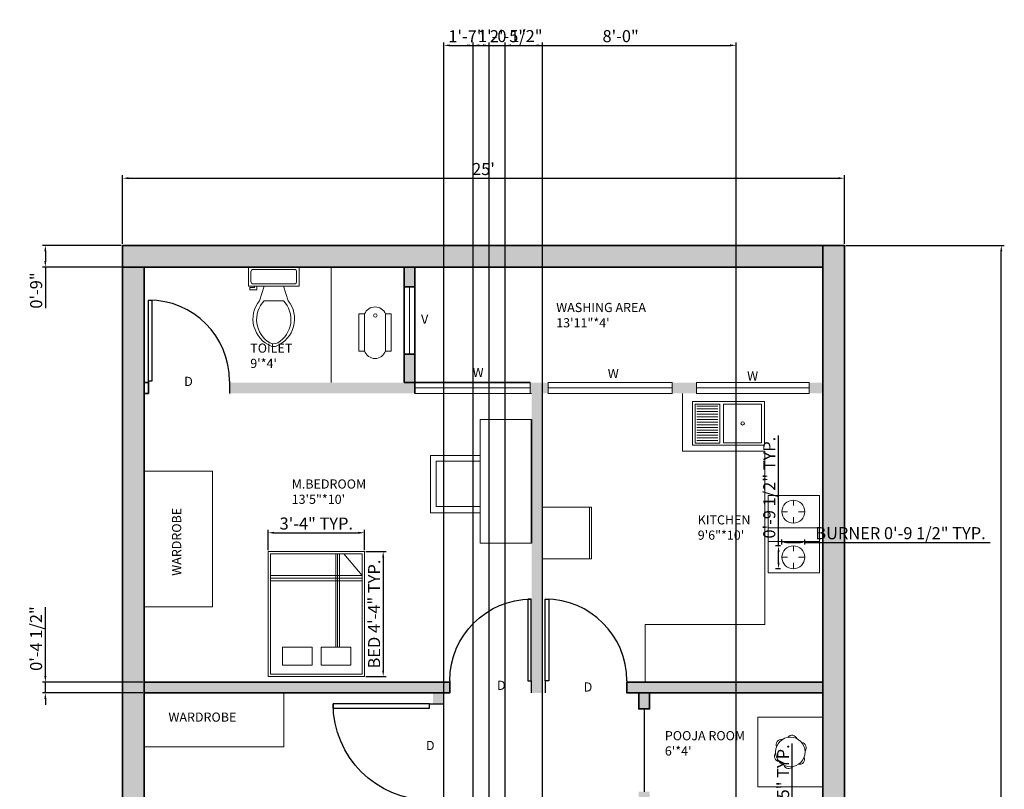
# Model space of a CAD drawing. Units: inches. Extents: x 2318 to 2727, y 1180 to 1889.
# Tile 2 of 2: x 2318 to 2727, y 1570 to 1889. Entities that reach past the tile are written whole.
import ezdxf

# ---------------------------------------------------------------- set-up
doc = ezdxf.new("R2010")
doc.units = ezdxf.units.IN
for name, color, linetype, lineweight in [('A-ANNO-DIMS', 2, 'Continuous', 18), ('A-ANNO-TEXT', 7, 'Continuous', 18), ('A-AREA-IDEN', 7, 'Continuous', 18), ('A-EQPM', 52, 'Continuous', 18), ('A-FIXT-PATT', 9, 'Continuous', 13), ('A-FLOR', 7, 'Continuous', 18), ('A-FLOR-CASE', 52, 'Continuous', 20), ('A-FLOR-FIXT', 9, 'Continuous', 18), ('A-FURN', 52, 'Continuous', 18), ('A-WALL-PATT', 192, 'Continuous', 13), ('BED', 52, 'Continuous', 18), ('DOOR', 20, 'Continuous', 25), ('WALL', 192, 'Continuous', 35), ('WIND', 130, 'Continuous', 20)]:
    doc.layers.add(name, color=color, linetype=linetype, lineweight=lineweight)
doc.styles.get("Standard").update_dxf_attribs({"font": 'arial.ttf'})
doc.dimstyles.new('ISO-25', dxfattribs={"dimtxt": 5, "dimasz": 2.5, "dimexe": 1.25, "dimexo": 0.625, "dimtad": 1, "dimdec": 0, "dimlunit": 4, "dimtxsty": 'Standard', "dimcen": 2.5, "dimadec": 0, "dimazin": 0, "dimtfac": 1, "dimtdec": 0, "dimtmove": 0, "dimatfit": 3, "dimfxl": 1, "dimarcsym": 0})

# ---------------------------------------------------------------- blocks, each defined once
blk = doc.blocks.new('*U2')
for p, q in [((0, 0), (-1e-16, -5.999999999999999)), ((40, -6e-16), (40, -6))]:
    blk.add_line(p, q)
blk.add_lwpolyline([(0, 0), (5.6e-15, 40), (1.750000000000007, 40), (1.749999999999998, -7e-16)], close=True)
blk.add_arc((0, 0), 40, 0, 90)
blk = doc.blocks.new('*U7')
blk.add_arc((-0.1440628503678454, -1.424150322514833), 2.132686200397339, 19.60574678084591, 143.7964675693192)
blk = doc.blocks.new('*U8')
at = {"layer": 'A-FLOR-CASE', "transparency": 16777216}
blk.add_blockref('*U7', (2638.812211336774, 1591.333415691406), dxfattribs=at)
for p, rotation in [((2632.993530862629, 1588.949941904776), 60), ((2643.785700422321, 1587.486027477606), 300), ((2632.148339474031, 1582.719079904348), 120), ((2642.940509033724, 1581.255165477177), 239.9999999999999), ((2637.121828559579, 1578.871691690548), 180)]:
    blk.add_blockref('*U7', p, dxfattribs=dict(at, rotation=rotation))
blk = doc.blocks.new('*U4')
for p, q in [((9.5, -6), (9.5, -2)), ((-8, -8.5), (-8, -8)), ((-7, -8), (-7, -9.5)), ((-4, -8), (-6, -14)), ((4, -8), (6, -14)), ((-10, -8.5), (-8, -8.5)), ((-10, -9.5), (-10, -8.5)), ((-7, -9.5), (-10, -9.5)), ((4, -14), (-4, -14))]:
    blk.add_line(p, q)
blk.add_lwpolyline([(10.5, -8), (10.5, 0), (-10.5, 0), (-10.5, -8)], close=True)
for points in [[(-9.5, -2), (-9.5, -6)], [(8.5, -1), (-8.5, -1)], [(-8.5, -7), (8.5, -7)]]:
    blk.add_lwpolyline(points)
for centre, radius, start, end in [((-8.625, -1.875), 0.8838834999999999, 81.86989999999999, 188.1300999999999), ((8.625, -1.875), 0.8838834999999999, 351.8699, 98.13009999999993), ((-8.625, -6.125), 0.8838834999999999, 171.869898, 278.1301), ((8.625, -6.125), 0.8838834999999999, 261.8699, 8.130099999999993), ((3.519562435188956, -21.58049502388982), 12.16902005083646, 141.4691096810948, 247.9714346835576), ((4.199957580658807, -21.81740929088453), 11.3291791325804, 136.3677254423718, 238.946823937405), ((-3.519499936778316, -21.58047137067522), 12.16903423757823, 292.0284332733152, 38.53070636800453), ((-4.199890672038477, -21.81738596564128), 11.32918622148567, 301.0530065773863, 43.63209216694732), ((2.09660981727e-05, -27.87646475467881), 4, 245.7318247449371, 294.2681740488959), ((2.09415214183e-05, -28.99996806116075), 4, 254.8605283244437, 285.1394707718433)]:
    blk.add_arc(centre, radius, start, end)
blk = doc.blocks.new('*D10')
at = {"layer": 'A-ANNO-DIMS', "color": 0, "lineweight": -2, "transparency": 16777216}
for p, q in [((2661.05912290835, 1795.62046240872), (2726.896794992849, 1795.62046240872)), ((2725.646794992849, 1216.12046240872), (2725.646794992849, 1793.12046240872)), ((2661.05912290835, 1213.62046240872), (2726.896794992849, 1213.62046240872))]:
    blk.add_line(p, q, dxfattribs=at)
at = {"layer": 'A-ANNO-DIMS', "color": 0, "transparency": 16777216}
for points in [[(2725.230128326182, 1793.12046240872), (2726.063461659516, 1793.12046240872), (2725.646794992849, 1795.62046240872)], [(2725.230128326182, 1216.12046240872), (2726.063461659516, 1216.12046240872), (2725.646794992849, 1213.62046240872)]]:
    blk.add_solid(points, dxfattribs=at)
at = {"layer": 'Defpoints', "color": 0, "transparency": 16777216}
for p in [(2660.434122908351, 1795.62046240872), (2725.646794992849, 1795.62046240872), (2660.434122908351, 1213.62046240872)]:
    blk.add_point(p, dxfattribs=at)
at = {"layer": 'A-ANNO-DIMS', "color": 0, "transparency": 16777216, "insert": (2722.468930054241, 1504.620462408719), "char_height": 5, "attachment_point": 5, "rotation": 90}
blk.add_mtext('48\'-6"', dxfattribs=at)
blk = doc.blocks.new('*D11')
at = {"layer": 'A-ANNO-DIMS', "color": 0, "lineweight": -2, "transparency": 16777216}
for p, q in [((2360.434122908349, 1796.24546240872), (2360.434122908349, 1824.759731731843)), ((2362.934122908349, 1823.509731731843), (2657.934122908349, 1823.509731731843)), ((2660.43412290835, 1796.24546240872), (2660.43412290835, 1824.759731731843))]:
    blk.add_line(p, q, dxfattribs=at)
at = {"layer": 'A-ANNO-DIMS', "color": 0, "transparency": 16777216}
for points in [[(2362.934122908349, 1823.92639839851), (2362.934122908349, 1823.093065065176), (2360.434122908349, 1823.509731731843)], [(2657.934122908349, 1823.92639839851), (2657.934122908349, 1823.093065065176), (2660.43412290835, 1823.509731731843)]]:
    blk.add_solid(points, dxfattribs=at)
at = {"layer": 'Defpoints', "color": 0, "transparency": 16777216}
for p in [(2660.43412290835, 1823.509731731843), (2360.434122908349, 1795.620462408719), (2660.43412290835, 1795.620462408719)]:
    blk.add_point(p, dxfattribs=at)
at = {"layer": 'A-ANNO-DIMS', "color": 0, "transparency": 16777216, "insert": (2510.43412290835, 1826.687596670451), "char_height": 5, "attachment_point": 5}
blk.add_mtext("25'", dxfattribs=at)
blk = doc.blocks.new('BED-DOUBLE')
for p, q in [((1.000105627843367, 31.46413777485918), (10.01316039580524, 39.02973591941259)), ((10.01316039580524, 39.02973591941259), (10.01316039580524, 0.9997279856868317)), ((11.11310554679403, 39.02973591941259), (11.11310554679403, 0.9997279856868317)), ((12.24178663289422, 39.02973591941259), (12.24178663289422, 0.9997279856868317)), ((39.71798243829289, 29.5953397455512), (1.000105627843367, 29.5953397455512)), ((1.000105627843367, 28.7976345667164), (39.71798243829289, 28.7976345667164)), ((39.71798243829289, 28.17233428248915), (1.000105627843367, 28.17233428248915))]:
    blk.add_line(p, q)
for points in [[(51.95742790868099, 40.02973591941258), (0.000105627843368, 40.02973591941258), (0.000105627843368, -0.0002720143131683), (51.95742790868099, -0.0002720143131683)], [(50.95742790868098, 39.02973591941259), (1.000105627843367, 39.02973591941259), (1.000105627843367, 0.9997279856868317), (50.95742790868098, 0.9997279856868317)], [(47.17675068467542, 34.33746874252188), (39.71798243829289, 34.33746874252188), (39.71798243829289, 22.00719982245642), (47.17675068467542, 22.00719982245642)], [(47.17675068467542, 18.28102639524536), (39.71798243829289, 18.28102639524536), (39.71798243829289, 5.950757475179898), (47.17675068467542, 5.950757475179898)]]:
    blk.add_lwpolyline(points, close=True)
blk = doc.blocks.new('WC-SQUAT')
for points in [[(-0.0004322986737861, 2.896310993941142), (2.391962376819265, 2.896310993941142), (2.391962376819265, 18.33525324847665), (-0.0004322986737861, 18.33525324847665)], [(11.06341502906935, 2.896310993941142), (13.4558097045624, 2.896310993941142), (13.4558097045624, 18.33525324847665), (11.06341502906935, 18.33525324847665)]]:
    blk.add_lwpolyline(points, close=True)
for points in [[(2.391962376819265, 18.28462303204901), (2.391962376819265, 2.896310993941142)], [(11.06341502906935, 2.896310993941142), (11.06341502906935, 18.28462303204901)]]:
    blk.add_lwpolyline(points)
blk.add_circle((6.600496095508333, 3.601330784865922), 0.7261776368631928)
for centre, radius, start, end in [((6.727688702944305, 16.89122133365617), 4.554129013119609, 17.81619851304262, 162.1838014869574), ((6.727688702944305, 4.693529829720773), 4.693454838254528, 202.5146865328957, 337.4853134671043)]:
    blk.add_arc(centre, radius, start, end)
blk = doc.blocks.new('COOKTOP-BURNER')
for p, q in [((4.735360270604815, 9.470945517394512), (4.735360270604815, 7.287879564605873)), ((-0.0002473178587934, 4.735337928930903), (2.36755647637301, 4.735337928930903)), ((9.470967859068423, 4.735337928930903), (6.916233003425531, 4.735337928930903)), ((4.735360270604815, -0.0002696595327052), (4.735360270604815, 2.431821280725898))]:
    blk.add_line(p, q)
blk.add_circle((4.735360270604815, 4.735337928930903), 4.735607588463608)
blk = doc.blocks.new('*D17')
at = {"layer": 'A-ANNO-DIMS', "color": 0, "lineweight": -2, "transparency": 16777216}
for p, q in [((2638.784887214313, 1554.866008932733), (2638.784887214313, 1588.622830215134)), ((2632.917587175159, 1554.866008932733), (2640.034887214313, 1554.866008932733)), ((2638.784887214313, 1540.504913553941), (2638.784887214313, 1552.366008932733)), ((2632.917587175159, 1538.004913553941), (2640.034887214313, 1538.004913553941))]:
    blk.add_line(p, q, dxfattribs=at)
at = {"layer": 'A-ANNO-DIMS', "color": 0, "transparency": 16777216}
for points in [[(2638.368220547646, 1552.366008932733), (2639.20155388098, 1552.366008932733), (2638.784887214313, 1554.866008932733)], [(2638.368220547646, 1540.504913553941), (2639.20155388098, 1540.504913553941), (2638.784887214313, 1538.004913553941)]]:
    blk.add_solid(points, dxfattribs=at)
at = {"layer": 'Defpoints', "color": 0, "transparency": 16777216}
for p in [(2632.292587175159, 1554.866008932733), (2638.784887214313, 1554.866008932733), (2632.292587175159, 1538.004913553941)]:
    blk.add_point(p, dxfattribs=at)
at = {"layer": 'A-ANNO-DIMS', "color": 0, "transparency": 16777216, "insert": (2635.607022275705, 1572.994419573932), "char_height": 5, "attachment_point": 5, "rotation": 90}
blk.add_mtext('1\'-5" TYP.', dxfattribs=at)
blk = doc.blocks.new('*D18')
at = {"layer": 'A-ANNO-DIMS', "color": 0, "lineweight": -2, "transparency": 16777216}
for p, q in [((2461.585850961747, 1668.391564033391), (2470.004449303873, 1668.391564033391)), ((2468.754449303873, 1665.891564033391), (2468.754449303873, 1618.934241752553)), ((2461.585850961747, 1616.434241752553), (2470.004449303873, 1616.434241752553))]:
    blk.add_line(p, q, dxfattribs=at)
at = {"layer": 'A-ANNO-DIMS', "color": 0, "transparency": 16777216}
for points in [[(2468.337782637207, 1665.891564033391), (2469.17111597054, 1665.891564033391), (2468.754449303873, 1668.391564033391)], [(2468.337782637207, 1618.934241752553), (2469.17111597054, 1618.934241752553), (2468.754449303873, 1616.434241752553)]]:
    blk.add_solid(points, dxfattribs=at)
at = {"layer": 'Defpoints', "color": 0, "transparency": 16777216}
for p in [(2460.960850961747, 1668.391564033391), (2460.960850961747, 1616.434241752553), (2468.754449303873, 1616.434241752553)]:
    blk.add_point(p, dxfattribs=at)
at = {"layer": 'A-ANNO-DIMS', "color": 0, "transparency": 16777216, "insert": (2465.627743983273, 1642.412902892971), "char_height": 5, "attachment_point": 5, "rotation": 90}
blk.add_mtext('BED 4\'-4" TYP.', dxfattribs=at)
blk = doc.blocks.new('*D19')
at = {"layer": 'A-ANNO-DIMS', "color": 0, "lineweight": -2, "transparency": 16777216}
for p, q in [((2420.93084302802, 1669.016564033389), (2420.93084302802, 1677.435162375515)), ((2423.43084302802, 1676.185162375515), (2458.460850961746, 1676.185162375515)), ((2460.960850961745, 1669.01656403339), (2460.960850961745, 1677.435162375515))]:
    blk.add_line(p, q, dxfattribs=at)
at = {"layer": 'A-ANNO-DIMS', "color": 0, "transparency": 16777216}
for points in [[(2423.43084302802, 1676.601829042182), (2423.43084302802, 1675.768495708849), (2420.93084302802, 1676.185162375515)], [(2458.460850961746, 1676.601829042182), (2458.460850961746, 1675.768495708849), (2460.960850961745, 1676.185162375515)]]:
    blk.add_solid(points, dxfattribs=at)
at = {"layer": 'Defpoints', "color": 0, "transparency": 16777216}
for p in [(2460.960850961745, 1676.185162375515), (2420.93084302802, 1668.391564033389), (2460.960850961745, 1668.39156403339)]:
    blk.add_point(p, dxfattribs=at)
at = {"layer": 'A-ANNO-DIMS', "color": 0, "transparency": 16777216, "insert": (2440.945846994883, 1679.364732634724), "char_height": 5, "attachment_point": 5}
blk.add_mtext('3\'-4" TYP.', dxfattribs=at)
blk = doc.blocks.new('*D22')
at = {"layer": 'A-ANNO-DIMS', "color": 0, "lineweight": -2, "transparency": 16777216}
for p, q in [((2634.483752682141, 1671.360651861982), (2634.483752682141, 1673.406334138521)), ((2636.983752682141, 1672.156334138521), (2641.454967859069, 1672.156334138521)), ((2643.954967859068, 1671.360651861982), (2643.954967859068, 1673.406334138521)), ((2643.954967859068, 1672.156334138521), (2721.047396235603, 1672.156334138521))]:
    blk.add_line(p, q, dxfattribs=at)
at = {"layer": 'A-ANNO-DIMS', "color": 0, "transparency": 16777216}
for points in [[(2636.983752682141, 1672.573000805188), (2636.983752682141, 1671.739667471855), (2634.483752682141, 1672.156334138521)], [(2641.454967859069, 1672.573000805188), (2641.454967859069, 1671.739667471855), (2643.954967859068, 1672.156334138521)]]:
    blk.add_solid(points, dxfattribs=at)
at = {"layer": 'Defpoints', "color": 0, "transparency": 16777216}
for p in [(2634.483752682141, 1670.735651861982), (2643.954967859068, 1672.156334138521), (2643.954967859068, 1670.735651861982)]:
    blk.add_point(p, dxfattribs=at)
at = {"layer": 'A-ANNO-DIMS', "color": 0, "transparency": 16777216, "insert": (2683.751182047336, 1675.366600168535), "char_height": 5, "attachment_point": 5}
blk.add_mtext('BURNER 0\'-9 1/2" TYP.', dxfattribs=at)
blk = doc.blocks.new('*D23')
at = {"layer": 'A-ANNO-DIMS', "color": 0, "lineweight": -2, "transparency": 16777216}
for p, q in [((2633.063070405604, 1670.735651861983), (2633.063070405604, 1716.613891971124)), ((2633.858752682142, 1670.735651861983), (2631.813070405604, 1670.735651861983)), ((2633.063070405604, 1663.764436685056), (2633.063070405604, 1668.235651861983)), ((2633.858752682142, 1661.264436685056), (2631.813070405604, 1661.264436685056))]:
    blk.add_line(p, q, dxfattribs=at)
at = {"layer": 'A-ANNO-DIMS', "color": 0, "transparency": 16777216}
for points in [[(2632.646403738938, 1668.235651861983), (2633.479737072271, 1668.235651861983), (2633.063070405604, 1670.735651861983)], [(2632.646403738938, 1663.764436685056), (2633.479737072271, 1663.764436685056), (2633.063070405604, 1661.264436685056)]]:
    blk.add_solid(points, dxfattribs=at)
at = {"layer": 'Defpoints', "color": 0, "transparency": 16777216}
for p in [(2633.063070405604, 1670.735651861983), (2634.483752682142, 1670.735651861983), (2634.483752682142, 1661.264436685056)]:
    blk.add_point(p, dxfattribs=at)
at = {"layer": 'A-ANNO-DIMS', "color": 0, "transparency": 16777216, "insert": (2629.85280437559, 1694.924771916552), "char_height": 5, "attachment_point": 5, "rotation": 90}
blk.add_mtext('0\'-9 1/2" TYP.', dxfattribs=at)
blk = doc.blocks.new('*D24')
at = {"layer": 'A-ANNO-DIMS', "color": 0, "lineweight": -2, "transparency": 16777216}
for p, q in [((2519.434123, 1223.245462), (2519.434123, 1879.970462)), ((2521.934123, 1878.720462), (2612.934123, 1878.720462)), ((2615.434123, 1223.245462), (2615.434123, 1879.970462))]:
    blk.add_line(p, q, dxfattribs=at)
at = {"layer": 'A-ANNO-DIMS', "color": 0, "transparency": 16777216}
for points in [[(2521.934123, 1879.137128666666), (2521.934123, 1878.303795333333), (2519.434123, 1878.720462)], [(2612.934123, 1879.137128666666), (2612.934123, 1878.303795333333), (2615.434123, 1878.720462)]]:
    blk.add_solid(points, dxfattribs=at)
at = {"layer": 'Defpoints', "color": 0, "transparency": 16777216}
for p in [(2615.434123, 1878.720462), (2519.434123, 1222.620462), (2615.434123, 1222.620462)]:
    blk.add_point(p, dxfattribs=at)
at = {"layer": 'A-ANNO-DIMS', "color": 0, "transparency": 16777216, "insert": (2567.434123, 1881.898326938608), "char_height": 5, "attachment_point": 5}
blk.add_mtext('8\'-0"', dxfattribs=at)
blk = doc.blocks.new('*D28')
at = {"layer": 'A-ANNO-DIMS', "color": 0, "lineweight": -2, "transparency": 16777216}
for p, q in [((2506.203301, 1386.745462), (2506.203301, 1879.970462)), ((2508.703301, 1878.720462), (2532.522673, 1878.720462)), ((2535.022673, 1386.745462), (2535.022673, 1879.970462))]:
    blk.add_line(p, q, dxfattribs=at)
at = {"layer": 'A-ANNO-DIMS', "color": 0, "transparency": 16777216}
for points in [[(2508.703301, 1879.137128666666), (2508.703301, 1878.303795333333), (2506.203301, 1878.720462)], [(2532.522673, 1879.137128666666), (2532.522673, 1878.303795333333), (2535.022673, 1878.720462)]]:
    blk.add_solid(points, dxfattribs=at)
at = {"layer": 'Defpoints', "color": 0, "transparency": 16777216}
for p in [(2535.022673, 1878.720462), (2506.203301, 1386.120462), (2535.022673, 1386.120462)]:
    blk.add_point(p, dxfattribs=at)
at = {"layer": 'A-ANNO-DIMS', "color": 0, "transparency": 16777216, "insert": (2520.612987, 1881.898326938608), "char_height": 5, "attachment_point": 5}
blk.add_mtext('2\'-5"', dxfattribs=at)
blk = doc.blocks.new('*D29')
at = {"layer": 'A-ANNO-DIMS', "color": 0, "lineweight": -2, "transparency": 16777216}
for p, q in [((2493.934123, 1386.745462), (2493.934123, 1879.970462)), ((2496.434123, 1878.720462), (2503.703301, 1878.720462)), ((2506.203301, 1386.745462), (2506.203301, 1879.970462)), ((2506.203301, 1878.720462), (2534.424651613916, 1878.720462))]:
    blk.add_line(p, q, dxfattribs=at)
at = {"layer": 'A-ANNO-DIMS', "color": 0, "transparency": 16777216}
for points in [[(2496.434123, 1879.137128666666), (2496.434123, 1878.303795333333), (2493.934123, 1878.720462)], [(2503.703301, 1879.137128666666), (2503.703301, 1878.303795333333), (2506.203301, 1878.720462)]]:
    blk.add_solid(points, dxfattribs=at)
at = {"layer": 'Defpoints', "color": 0, "transparency": 16777216}
for p in [(2506.203301, 1878.720462), (2493.934123, 1386.120462), (2506.203301, 1386.120462)]:
    blk.add_point(p, dxfattribs=at)
at = {"layer": 'A-ANNO-DIMS', "color": 0, "transparency": 16777216, "insert": (2521.563976306957, 1881.930728030013), "char_height": 5, "attachment_point": 5}
blk.add_mtext('1\'-0 1/2"', dxfattribs=at)
blk = doc.blocks.new('*D30')
at = {"layer": 'A-ANNO-DIMS', "color": 0, "lineweight": -2, "transparency": 16777216}
for p, q in [((2493.934123, 1310.245462), (2493.934123, 1879.970462)), ((2496.434123, 1878.720462), (2510.283342000001, 1878.720462)), ((2512.783342, 1317.956646), (2512.783342, 1879.970462))]:
    blk.add_line(p, q, dxfattribs=at)
at = {"layer": 'A-ANNO-DIMS', "color": 0, "transparency": 16777216}
for points in [[(2496.434123, 1879.137128666666), (2496.434123, 1878.303795333333), (2493.934123, 1878.720462)], [(2510.283342000001, 1879.137128666666), (2510.283342000001, 1878.303795333333), (2512.783342, 1878.720462)]]:
    blk.add_solid(points, dxfattribs=at)
at = {"layer": 'Defpoints', "color": 0, "transparency": 16777216}
for p in [(2512.783342, 1878.720462), (2512.783342, 1317.331646), (2493.934123, 1309.620462)]:
    blk.add_point(p, dxfattribs=at)
at = {"layer": 'A-ANNO-DIMS', "color": 0, "transparency": 16777216, "insert": (2503.3587325, 1881.855693923602), "char_height": 5, "attachment_point": 5}
blk.add_mtext('1\'-7"', dxfattribs=at)
blk = doc.blocks.new('*D33')
at = {"layer": 'A-ANNO-DIMS', "color": 0, "lineweight": -2, "transparency": 16777216}
for p, q in [((2359.809123000001, 1795.620462000001), (2327.084123000002, 1795.620462000001)), ((2328.334123000002, 1793.120462000001), (2328.334123000002, 1789.120462000001)), ((2368.809123000001, 1786.620462000001), (2327.084123000002, 1786.620462000001)), ((2328.334123000002, 1786.620462000001), (2328.334123000002, 1769.579193241474))]:
    blk.add_line(p, q, dxfattribs=at)
at = {"layer": 'A-ANNO-DIMS', "color": 0, "transparency": 16777216}
for points in [[(2327.917456333335, 1793.120462000001), (2328.750789666669, 1793.120462000001), (2328.334123000002, 1795.620462000001)], [(2327.917456333335, 1789.120462000001), (2328.750789666669, 1789.120462000001), (2328.334123000002, 1786.620462000001)]]:
    blk.add_solid(points, dxfattribs=at)
at = {"layer": 'Defpoints', "color": 0, "transparency": 16777216}
for p in [(2360.434123000001, 1795.620462000001), (2328.334123000002, 1786.620462000001), (2369.434123000001, 1786.620462000001)]:
    blk.add_point(p, dxfattribs=at)
at = {"layer": 'A-ANNO-DIMS', "color": 0, "transparency": 16777216, "insert": (2325.156258061394, 1776.849827620736), "char_height": 5, "attachment_point": 5, "rotation": 90}
blk.add_mtext('0\'-9"', dxfattribs=at)
blk = doc.blocks.new('*D34')
at = {"layer": 'A-ANNO-DIMS', "color": 0, "lineweight": -2, "transparency": 16777216}
for p, q in [((2328.334123000002, 1616.620462000001), (2328.334123000002, 1645.312481099592)), ((2368.809123000001, 1614.120462000001), (2327.084123000002, 1614.120462000001)), ((2328.334123000002, 1609.620462000001), (2328.334123000002, 1614.120462000001)), ((2368.809123000001, 1609.620462000001), (2327.084123000002, 1609.620462000001)), ((2328.334123000002, 1607.120462000001), (2328.334123000002, 1604.620462000001))]:
    blk.add_line(p, q, dxfattribs=at)
at = {"layer": 'A-ANNO-DIMS', "color": 0, "transparency": 16777216}
for points in [[(2327.917456333335, 1616.620462000001), (2328.750789666669, 1616.620462000001), (2328.334123000002, 1614.120462000001)], [(2327.917456333335, 1607.120462000001), (2328.750789666669, 1607.120462000001), (2328.334123000002, 1609.620462000001)]]:
    blk.add_solid(points, dxfattribs=at)
at = {"layer": 'Defpoints', "color": 0, "transparency": 16777216}
for p in [(2328.334123000002, 1614.120462000001), (2369.434123000001, 1614.120462000001), (2369.434123000001, 1609.620462000001)]:
    blk.add_point(p, dxfattribs=at)
at = {"layer": 'A-ANNO-DIMS', "color": 0, "transparency": 16777216, "insert": (2325.123856969988, 1632.216471549795), "char_height": 5, "attachment_point": 5, "rotation": 90}
blk.add_mtext('0\'-4 1/2"', dxfattribs=at)

msp = doc.modelspace()

# ---------------------------------------------------------------- hatches: boundary and pattern name
at = {"layer": 'A-FIXT-PATT'}
h = msp.add_hatch(dxfattribs=at)
h.set_pattern_fill('ANSI31', color=256, scale=0.3454888316707821, angle=-45, style=0)
h.set_pattern_definition([(0, (0, 0), (0, 1.096927040554733), [])])
h.paths.add_polyline_path([(2599.064826425526, 1714.495964387048), (2607.794309831661, 1714.495964387048), (2607.794309831661, 1728.758015914259), (2599.064826425526, 1728.758015914259)])
at = {"layer": 'A-WALL-PATT'}
h = msp.add_hatch(color=256, dxfattribs=at)
h.dxf.hatch_style = 1
h.paths.add_polyline_path([(2651.43412290835, 1795.620462408719), (2360.434122908349, 1795.620462408719), (2360.434122908349, 1786.620462408719), (2369.43412290835, 1786.620462408719), (2651.43412290835, 1786.620462408719)])
h.paths.add_polyline_path([(2481.93412290835, 1786.620462408719), (2477.434122908349, 1786.620462408719), (2477.434122908349, 1778.409720863707), (2481.93412290835, 1778.409720863707)])
h.paths.add_polyline_path([(2481.93412290835, 1750.357662348155), (2477.434122908349, 1750.357662348155), (2477.434122908349, 1738.620462408719), (2481.93412290835, 1738.620462408719)])
h.paths.add_polyline_path([(2369.43412290835, 1786.620462408719), (2360.434122908349, 1786.620462408719), (2360.434122908349, 1213.620462408719), (2369.43412290835, 1213.620462408719)])
h.paths.add_polyline_path([(2660.43412290835, 1795.620462408719), (2651.43412290835, 1795.620462408719), (2651.43412290835, 1786.620462408719), (2651.43412290835, 1213.620462408719), (2660.43412290835, 1213.620462408719)])
h.paths.add_polyline_path([(2496.406356271093, 1614.120462408719), (2369.43412290835, 1614.120462408719), (2369.43412290835, 1609.620462408719), (2496.406356271093, 1609.620462408719)])
h.paths.add_polyline_path([(2651.43412290835, 1614.120462408719), (2570.029056558353, 1614.120462408719), (2570.029056558353, 1609.620462408719), (2651.43412290835, 1609.620462408719)])
h.paths.add_polyline_path([(2579.434122908349, 1609.620462408719), (2574.934122908349, 1609.620462408719), (2574.934122908349, 1602.977157394022), (2579.434122908349, 1602.977157394022)])
h.paths.add_polyline_path([(2579.434122908349, 1568.53500508798), (2574.934122908349, 1568.53500508798), (2574.934122908349, 1557.120462408719), (2579.434122908349, 1557.120462408719)])
h.paths.add_polyline_path([(2651.43412290835, 1561.620462408719), (2579.434122908349, 1561.620462408719), (2579.434122908349, 1557.120462408719), (2651.43412290835, 1557.120462408719)])
h.paths.add_polyline_path([(2493.93412290835, 1565.110264395277), (2489.434122908349, 1565.110264395277), (2489.434122908349, 1436.361954917535), (2493.93412290835, 1436.361954917535)])
h.paths.add_polyline_path([(2489.434122908349, 1419.398753224193), (2432.93412290835, 1419.398753224193), (2432.93412290835, 1411.620462408719), (2489.434122908349, 1411.620462408719)])
h.paths.add_polyline_path([(2493.93412290835, 1397.391843110563), (2489.434122908349, 1397.391843110563), (2489.434122908349, 1309.620462408719), (2493.93412290835, 1309.620462408719)])
h.paths.add_polyline_path([(2506.203300764954, 1386.120462408719), (2493.93412290835, 1386.120462408719), (2493.93412290835, 1381.620462408719), (2506.203300764954, 1381.620462408719)])
h.paths.add_polyline_path([(2651.43412290835, 1434.120462408719), (2536.93412290835, 1434.120462408719), (2536.93412290835, 1429.620462408719), (2651.43412290835, 1429.620462408719)])
h.paths.add_polyline_path([(2541.434122908349, 1429.620462408719), (2536.934122908349, 1429.620462408719), (2536.934122908349, 1427.358325609929), (2541.434122908349, 1427.358325609929)])
h.paths.add_polyline_path([(2541.434122908349, 1387.358325609929), (2536.934122908349, 1387.358325609929), (2536.934122908349, 1309.62046240872), (2541.434122908349, 1309.62046240872)])
h.paths.add_polyline_path([(2536.934122908349, 1386.120462408719), (2535.022673263742, 1386.120462408719), (2535.022673263742, 1381.797556533901), (2535.022673263742, 1381.620462408719), (2536.934122908349, 1381.620462408719)])
h.paths.add_polyline_path([(2536.934122908349, 1309.620462408719), (2489.434122908349, 1309.620462408719), (2489.434122908349, 1305.120462408719), (2536.934122908349, 1305.120462408719)])
h.paths.add_polyline_path([(2651.43412290835, 1309.620462408719), (2536.934122908349, 1309.620462408719), (2536.934122908349, 1305.120462408719), (2651.43412290835, 1305.120462408719)])
h.paths.add_polyline_path([(2651.43412290835, 1222.620462408719), (2638.898654194149, 1222.620462408719), (2638.898654194149, 1213.620462408719), (2651.43412290835, 1213.620462408719)])
h.paths.add_polyline_path([(2588.93760602221, 1222.620462408719), (2489.587992845893, 1222.620462408719), (2489.587992845893, 1213.620462408719), (2588.93760602221, 1213.620462408719)])
h = msp.add_hatch(color=256, dxfattribs=at)
h.dxf.hatch_style = 1
h.paths.add_polyline_path([(2481.93412290835, 1738.620462408719), (2477.434122908349, 1738.620462408719), (2404.898801810678, 1738.620462408719), (2404.898801810678, 1734.120462408719), (2481.93412290835, 1734.120462408719)])
h.paths.add_polyline_path([(2537.328192578414, 1738.620462408719), (2529.859535196069, 1738.620462408719), (2529.859535196069, 1734.12046240872), (2530.43412290835, 1734.12046240872), (2530.43412290835, 1614.120462408719), (2534.934122908349, 1614.120462408719), (2534.934122908349, 1734.120462408719), (2537.328192578414, 1734.120462408719)])
h.paths.add_polyline_path([(2598.995804292892, 1738.620462408719), (2588.850327023185, 1738.620462408719), (2588.850327023185, 1734.120462408719), (2598.995804292892, 1734.120462408719)])
h.paths.add_polyline_path([(2651.43412290835, 1738.620462408719), (2645.813659683537, 1738.620462408719), (2645.813659683537, 1734.120462408719), (2651.43412290835, 1734.120462408719)])
h.paths.add_polyline_path([(2534.934122908349, 1614.120462408719), (2530.43412290835, 1614.120462408719), (2530.301674273302, 1614.120462408719), (2530.301674273302, 1609.620462408719), (2534.934122908349, 1609.620462408719)])
h.paths.add_polyline_path([(2493.93412290835, 1609.620462408719), (2489.434122908349, 1609.620462408719), (2489.434122908349, 1605.110264395277), (2493.93412290835, 1605.110264395277)])
h.paths.add_polyline_path([(2386.21635784955, 1416.120462408719), (2369.43412290835, 1416.120462408719), (2369.43412290835, 1411.620462408719), (2386.21635784955, 1411.620462408719)])
h.paths.add_polyline_path([(2432.93412290835, 1416.120462408719), (2432.93412290835, 1485.120462408719), (2428.434122908349, 1485.120462408719), (2428.434122908349, 1416.120462408719), (2412.834170443626, 1416.120462408719), (2412.834170443626, 1411.620462408719), (2428.434122908349, 1411.620462408719), (2432.93412290835, 1411.620462408719)])
h = msp.add_hatch(dxfattribs=at)
h.set_pattern_fill('ANGLE', color=256)
h.set_pattern_definition([(0, (0, 0), (0, 6.985), [5.08, -1.905]), (90, (0, 0), (-6.985, 4e-16), [5.08, -1.905])])
h.paths.add_polyline_path([(2371.176239539582, 1738.620462408719), (2369.43412290835, 1738.620462408719), (2369.43412290835, 1734.120462408719), (2371.176239539582, 1734.120462408719)])

# ---------------------------------------------------------------- linework, layer by layer
at = {"layer": 'A-EQPM'}
msp.add_line((2554.451565274374, 1665.290601360766), (2554.451565274374, 1686.754229428795), dxfattribs=at)
for points in [[(2628.72816688043, 1659.535164210019), (2650.08408976813, 1659.535164210019), (2650.08408976813, 1691.713782306337), (2628.72816688043, 1691.713782306337)], [(2534.934122908349, 1665.290601360766), (2555.365448738543, 1665.290601360766), (2555.365448738543, 1686.754229428795), (2534.934122908349, 1686.754229428795)], [(2628.72816688043, 1672.523135203119), (2650.08408976813, 1672.523135203119), (2650.08408976813, 1678.281503882785), (2628.72816688043, 1678.281503882785)]]:
    msp.add_lwpolyline(points, close=True, dxfattribs=at)
at = {"layer": 'A-FLOR'}
msp.add_line((2447.155356034822, 1738.620462408719), (2447.155356034822, 1786.620462408719), dxfattribs=at)
at = {"layer": 'A-FLOR-CASE'}
for p, q in [((2593.184122908349, 1734.120462408719), (2593.184122908349, 1710.120462408719)), ((2593.184122908349, 1710.120462408719), (2627.434122908349, 1710.120462408719)), ((2627.434122908349, 1638.12046240872), (2627.434122908349, 1710.120462408719)), ((2577.648264660169, 1614.120462408719), (2577.648264660169, 1638.12046240872)), ((2577.648264660169, 1638.12046240872), (2627.434122908349, 1638.12046240872))]:
    msp.add_line(p, q, dxfattribs=at)
for points in [[(2369.43412290835, 1645.433057256802), (2397.734065286946, 1645.433057256802), (2397.734065286946, 1701.828758101606), (2369.43412290835, 1701.828758101606)], [(2369.43412290835, 1609.620462408719), (2427.45459817024, 1609.620462408719), (2427.45459817024, 1587.177172170308), (2369.43412290835, 1587.177172170308)], [(2651.43412290835, 1599.574104316289), (2624.499916988003, 1599.574104316289), (2624.499916988003, 1570.631003065665), (2651.43412290835, 1570.631003065665)]]:
    msp.add_lwpolyline(points, close=True, dxfattribs=at)
msp.add_circle((2637.967019948176, 1585.102553690977), 6.151512465651569, dxfattribs=at)
at = {"layer": 'A-FLOR-FIXT'}
for points in [[(2597.371051855882, 1712.570280403749), (2627.265413083551, 1712.570280403749), (2627.265413083551, 1730.780841195242), (2597.371051855882, 1730.780841195242)], [(2598.448144874791, 1729.670172704353), (2608.680528554411, 1729.670172704353), (2608.680528554411, 1713.467877107661), (2598.448144874791, 1713.467877107661)], [(2610.23919299803, 1729.670172704353), (2626.036552100492, 1729.670172704353), (2626.036552100492, 1713.5876113384), (2610.23919299803, 1713.5876113384)]]:
    msp.add_lwpolyline(points, close=True, dxfattribs=at)
msp.add_circle((2618.137872549261, 1721.628892021377), 0.7179248791135251, dxfattribs=at)
at = {"layer": 'A-FURN'}
for p, q in [((2488.426058181723, 1684.474029412591), (2488.426058181723, 1708.335196138952)), ((2488.426058181723, 1708.335196138952), (2509.058537214118, 1708.335196138952)), ((2509.058537214118, 1684.474029412591), (2488.426058181723, 1684.474029412591))]:
    msp.add_line(p, q, dxfattribs=at)
for points in [[(2530.43412290835, 1723.268707939353), (2509.058537214118, 1723.268707939353), (2509.058537214118, 1671.813001379365), (2530.43412290835, 1671.813001379365)], [(2509.058537214118, 1705.900380572135), (2490.700512879346, 1705.900380572135), (2490.700512879346, 1687.071163864825), (2509.058537214118, 1687.071163864825)]]:
    msp.add_lwpolyline(points, close=True, dxfattribs=at)
at = {"layer": 'DOOR'}
msp.add_line((2577.184122908349, 1602.977157394022), (2577.184122908347, 1568.53500508798), dxfattribs=at)
at = {"layer": 'WALL'}
for p, q in [((2360.434122908349, 1795.620462408719), (2660.43412290835, 1795.620462408719)), ((2360.434122908349, 1213.620462408719), (2360.434122908349, 1795.620462408719)), ((2660.43412290835, 1795.620462408719), (2660.43412290835, 1213.620462408719)), ((2369.43412290835, 1786.620462408719), (2477.434122908349, 1786.620462408719)), ((2477.434122908349, 1786.620462408719), (2477.434122908349, 1738.620462408719)), ((2481.93412290835, 1786.620462408719), (2481.93412290835, 1734.120462408719)), ((2481.93412290835, 1786.620462408719), (2637.93412290835, 1786.620462408719)), ((2371.176239539581, 1738.620462408719), (2369.43412290835, 1738.620462408719)), ((2477.434122908349, 1738.620462408719), (2529.859535196069, 1738.620462408719)), ((2369.43412290835, 1734.120462408719), (2369.43412290835, 1614.120462408719)), ((2371.176239539582, 1734.120462408719), (2369.43412290835, 1734.120462408719)), ((2530.43412290835, 1671.813001379365), (2530.43412290835, 1723.268707939353)), ((2369.43412290835, 1614.120462408719), (2496.406356271093, 1614.120462408719)), ((2530.301674273302, 1614.120462408719), (2530.43412290835, 1614.120462408719)), ((2570.029056558353, 1614.120462408719), (2651.43412290835, 1614.120462408719)), ((2369.43412290835, 1609.620462408719), (2496.406356271093, 1609.620462408719)), ((2369.43412290835, 1609.620462408719), (2489.434122908349, 1609.620462408719)), ((2570.029056558353, 1609.620462408719), (2651.43412290835, 1609.620462408719)), ((2574.934122908349, 1602.977157394022), (2574.934122908349, 1609.620462408719)), ((2579.434122908349, 1602.977157394022), (2579.434122908349, 1609.620462408719)), ((2651.43412290835, 1609.620462408719), (2651.43412290835, 1561.620462408719)), ((2574.934122908349, 1602.977157394022), (2579.434122908349, 1602.977157394022))]:
    msp.add_line(p, q, dxfattribs=at)
for points in [[(2369.43412290835, 1213.620462408719), (2360.434122908349, 1213.620462408719), (2360.434122908349, 1795.620462408719), (2660.43412290835, 1795.620462408719), (2660.43412290835, 1213.620462408719), (2489.587992845893, 1213.620462408719)], [(2369.43412290835, 1222.620462408719), (2369.43412290835, 1786.620462408719), (2651.43412290835, 1786.620462408719), (2651.43412290835, 1222.620462408719), (2489.587992845893, 1222.620462408719)]]:
    msp.add_lwpolyline(points, dxfattribs=at)
for points in [[(2360.434122908349, 1795.620462408719), (2651.43412290835, 1795.620462408719), (2651.43412290835, 1786.620462408719), (2360.434122908349, 1786.620462408719)], [(2651.43412290835, 1795.620462408719), (2660.43412290835, 1795.620462408719), (2660.43412290835, 1213.620462408719), (2651.43412290835, 1213.620462408719)], [(2360.434122908349, 1213.620462408719), (2369.43412290835, 1213.620462408719), (2369.43412290835, 1786.620462408719), (2360.434122908349, 1786.620462408719)], [(2477.434122908349, 1786.620462408719), (2481.93412290835, 1786.620462408719), (2481.93412290835, 1778.409720863707), (2477.434122908349, 1778.409720863707)], [(2477.434122908349, 1738.620462408719), (2481.93412290835, 1738.620462408719), (2481.93412290835, 1750.357662348155), (2477.434122908349, 1750.357662348155)], [(2371.176239539582, 1738.620462408719), (2369.43412290835, 1738.620462408719), (2369.43412290835, 1734.120462408719), (2371.176239539582, 1734.120462408719)], [(2369.43412290835, 1614.120462408719), (2496.406356271093, 1614.120462408719), (2496.406356271093, 1609.620462408719), (2369.43412290835, 1609.620462408719)], [(2570.029056558353, 1614.120462408719), (2651.43412290835, 1614.120462408719), (2651.43412290835, 1609.620462408719), (2570.029056558353, 1609.620462408719)], [(2574.934122908349, 1609.620462408719), (2579.434122908349, 1609.620462408719), (2579.434122908349, 1602.977157394022), (2574.934122908349, 1602.977157394022)]]:
    msp.add_lwpolyline(points, close=True, dxfattribs=at)
at = {"layer": 'WIND'}
for p, q in [((2479.684122908349, 1750.357662348155), (2479.684122908349, 1778.409720863707)), ((2481.93412290835, 1736.370462408719), (2529.859535196069, 1736.370462408719)), ((2537.328192578414, 1734.120462408719), (2537.328192578414, 1738.620462408719)), ((2537.328192578414, 1738.620462408719), (2588.850327023185, 1738.620462408719)), ((2537.328192578414, 1736.370462408719), (2588.850327023185, 1736.370462408719)), ((2598.995804292892, 1738.620462408719), (2645.813659683537, 1738.620462408719)), ((2598.995804292892, 1736.370462408719), (2645.813659683537, 1736.370462408719)), ((2481.93412290835, 1734.120462408719), (2530.43412290835, 1734.12046240872)), ((2537.328192578414, 1734.120462408719), (2588.850327023185, 1734.120462408719)), ((2598.995804292892, 1734.120462408719), (2645.813659683537, 1734.120462408719))]:
    msp.add_line(p, q, dxfattribs=at)
for points in [[(2477.434122908349, 1750.357662348155), (2481.93412290835, 1750.357662348155), (2481.93412290835, 1778.409720863707), (2477.434122908349, 1778.409720863707)], [(2481.93412290835, 1734.120462408719), (2529.859535196069, 1734.120462408719), (2529.859535196069, 1738.62046240872), (2481.93412290835, 1738.62046240872)], [(2537.328192578414, 1734.120462408719), (2588.850327023185, 1734.120462408719), (2588.850327023185, 1738.620462408719), (2537.328192578414, 1738.620462408719)], [(2598.995804292892, 1738.620462408719), (2645.813659683537, 1738.620462408719), (2645.813659683537, 1734.12046240872), (2598.995804292892, 1734.12046240872)]]:
    msp.add_lwpolyline(points, close=True, dxfattribs=at)

# ---------------------------------------------------------------- block references
at = {"layer": 'A-EQPM'}
for p in [(2634.484, 1680.207), (2634.484, 1661.264706344588)]:
    msp.add_blockref('COOKTOP-BURNER', p, dxfattribs=at)
at = {"layer": 'A-FLOR-CASE'}
msp.add_blockref('*U8', (0, 0), dxfattribs=at)
at = {"layer": 'A-FLOR-FIXT'}
msp.add_blockref('*U4', (2423.28140251092, 1786.620462408719), dxfattribs=at)
at = {"layer": 'A-FLOR-FIXT', "rotation": 180}
msp.add_blockref('WC-SQUAT', (2472.08091785341, 1770.047578984617), dxfattribs=at)
at = {"layer": 'BED', "rotation": 270.0000000000004}
msp.add_blockref('BED-DOUBLE', (2420.931115042333, 1668.391669661233), dxfattribs=at)
at = {"layer": 'DOOR'}
for p, xscale, yscale, zscale in [((2371.176239539582, 1739.178846749384), 0.8430640567774181, 0.8430640567774181, 0.8430640567774181), ((2530.301674273302, 1614.70476010905), -0.847382950055209, 0.847382950055209, 0.847382950055209), ((2536.117635035385, 1614.707175637165), 0.8477855380742031, 0.8477855380742031, 0.8477855380742031)]:
    msp.add_blockref('*U2', p, dxfattribs=dict(at, xscale=xscale, yscale=yscale, zscale=zscale))
at = {"layer": 'DOOR', "xscale": -1, "rotation": 90}
msp.add_blockref('*U2', (2487.934122908349, 1605.110264395277), dxfattribs=at)

# ---------------------------------------------------------------- texts
at = {"layer": 'A-ANNO-TEXT', "char_height": 3.809518626736397, "attachment_point": 1}
for s, insert in [('V', (2484.486695968714, 1766.819667265833)), ('W', (2505.926721968547, 1744.699605927507)), ('W', (2562.09054224899, 1744.248275628494)), ('D', (2386.05190160665, 1741.000885939125)), ('W', (2620.009812165261, 1743.248323116077)), ('D', (2516.06595463692, 1614.703550042737)), ('D', (2552.083891873545, 1614.014143728895)), ('WARDROBE', (2379.480557035822, 1601.484717419889)), ('D', (2486.526411439794, 1589.698326505239))]:
    msp.add_mtext_dynamic_manual_height_columns(s, width=80.53964032626133, gutter_width=19.04759313368198, heights=[0], dxfattribs=dict(at, insert=insert))
at = {"layer": 'A-ANNO-TEXT', "insert": (2380.986261513813, 1658.312652658997), "char_height": 3.809518626736397, "attachment_point": 1, "rotation": 90}
msp.add_mtext_dynamic_manual_height_columns('WARDROBE', width=80.53964032626133, gutter_width=19.04759313368198, heights=[0], dxfattribs=at)
at = {"layer": 'A-AREA-IDEN', "char_height": 3.809518626736397, "attachment_point": 1}
for s, insert in [('WASHING AREA\\P13\'11"*4\'', (2540.660684606084, 1771.704559102459)), ("TOILET\\P9'*4'", (2413.495334014237, 1754.822224568161)), ('M.BEDROOM\\P13\'5"*10\'', (2430.714425998905, 1698.351246694062)), ('KITCHEN\\P9\'6"*10\'', (2599.483115373078, 1683.456754873439)), ("POOJA ROOM\\P6'*4'", (2585.819568953843, 1593.771544727054))]:
    msp.add_mtext_dynamic_manual_height_columns(s, width=80.53964032626133, gutter_width=19.04759313368198, heights=[0], dxfattribs=dict(at, insert=insert))

# ---------------------------------------------------------------- dimensions: what is measured, and where the dimension line sits
at = {"layer": 'A-ANNO-DIMS'}
for base, p1, p2, override, picture, middle in [((2506.203301, 1878.720462), (2493.934123, 1386.120462), (2506.203301, 1386.120462), {"dimdec": 1, "dimlfac": 1, "dimrnd": 0, "dimzin": 1, "dimdsep": 46, "dimlunit": 4, "dimfrac": 2}, '*D29', (2521.563976306957, 1881.930728030013)), ((2512.783342, 1878.720462), (2493.934123, 1309.620462), (2512.783342, 1317.331646), {"dimdec": 1, "dimlfac": 1, "dimrnd": 0, "dimzin": 1, "dimdsep": 46, "dimlunit": 4, "dimfrac": 2}, '*D30', (2503.3587325, 1881.855693923602)), ((2535.022673, 1878.720462), (2506.203301, 1386.120462), (2535.022673, 1386.120462), {"dimdec": 1, "dimlfac": 1, "dimrnd": 0, "dimzin": 1, "dimdsep": 46, "dimlunit": 4, "dimfrac": 2}, '*D28', (2520.612987, 1881.898326938608)), ((2615.434123, 1878.720462), (2519.434123, 1222.620462), (2615.434123, 1222.620462), {"dimdec": 1, "dimlfac": 1, "dimrnd": 0, "dimzin": 1, "dimdsep": 46, "dimlunit": 4, "dimfrac": 2}, '*D24', (2567.434123, 1881.898326938608)), ((2660.43412290835, 1823.509731731843), (2360.434122908349, 1795.620462408719), (2660.43412290835, 1795.620462408719), {"dimclrd": 0, "dimclre": 0, "dimclrt": 0}, '*D11', (2510.43412290835, 1826.687596670451))]:
    dim = msp.add_linear_dim(base=base, p1=p1, p2=p2, dimstyle='ISO-25', override=override, dxfattribs=at)
    dim.commit()
    dim.dimension.update_dxf_attribs({"geometry": picture, "text_midpoint": middle})
for base, p1, p2, override, picture, middle in [((2328.334123000002, 1786.620462000001), (2360.434123, 1795.620462), (2369.434123, 1786.620462), {"dimdec": 1, "dimlfac": 1, "dimrnd": 0, "dimzin": 1, "dimdsep": 46, "dimlunit": 4, "dimfrac": 2}, '*D33', (2325.156258061394, 1776.849827620736)), ((2725.646794992849, 1795.62046240872), (2660.43412290835, 1213.620462408719), (2660.43412290835, 1795.620462408719), {"dimclrd": 0, "dimclre": 0, "dimclrt": 0}, '*D10', (2722.468930054241, 1504.620462408719)), ((2328.334123000002, 1614.120462000001), (2369.434123, 1609.620462), (2369.434123, 1614.120462), {"dimdec": 1, "dimlfac": 1, "dimrnd": 0, "dimzin": 1, "dimdsep": 46, "dimlunit": 4, "dimfrac": 2}, '*D34', (2325.123856969988, 1632.216471549795))]:
    dim = msp.add_linear_dim(base=base, p1=p1, p2=p2, angle=90, dimstyle='ISO-25', override=override, dxfattribs=at)
    dim.commit()
    dim.dimension.update_dxf_attribs({"geometry": picture, "text_midpoint": middle})
for base, p1, p2, angle, text, picture, middle in [((2633.063070405604, 1670.735651861983), (2634.483752682141, 1661.264436685055), (2634.483752682141, 1670.735651861982), 90, '<> TYP.', '*D23', (2629.85280437559, 1694.924771916552)), ((2460.960850961745, 1676.185162375515), (2420.93084302802, 1668.391564033389), (2460.960850961745, 1668.39156403339), 3.254e-13, '<> TYP.', '*D19', (2440.945846994883, 1679.364732634724)), ((2468.754449303873, 1616.434241752553), (2460.960850961745, 1668.39156403339), (2460.960850961746, 1616.434241752552), 270.0000000000005, 'BED <> TYP.', '*D18', (2465.627743983273, 1642.412902892971)), ((2638.784887214313, 1554.866008932733), (2632.292587175158, 1538.00491355394), (2632.292587175158, 1554.866008932732), 90, '<> TYP.', '*D17', (2635.607022275705, 1572.994419573932))]:
    dim = msp.add_linear_dim(base=base, p1=p1, p2=p2, angle=angle, text=text, dimstyle='ISO-25', override={"dimdec": 1, "dimlfac": 1, "dimrnd": 0, "dimzin": 1, "dimdsep": 46, "dimlunit": 4, "dimfrac": 2}, dxfattribs=at)
    dim.commit()
    dim.dimension.update_dxf_attribs({"geometry": picture, "text_midpoint": middle})
dim = msp.add_linear_dim(base=(2643.954967859068, 1672.156334138521), p1=(2634.483752682141, 1670.735651861982), p2=(2643.954967859068, 1670.735651861982), text='BURNER <> TYP.', dimstyle='ISO-25', override={"dimdec": 1, "dimlfac": 1, "dimrnd": 0, "dimzin": 1, "dimdsep": 46, "dimlunit": 4, "dimfrac": 2}, dxfattribs=at)
dim.commit()
dim.dimension.update_dxf_attribs({"geometry": '*D22', "text_midpoint": (2683.751182047336, 1675.366600168535)})

doc.saveas('drawing.dxf')
